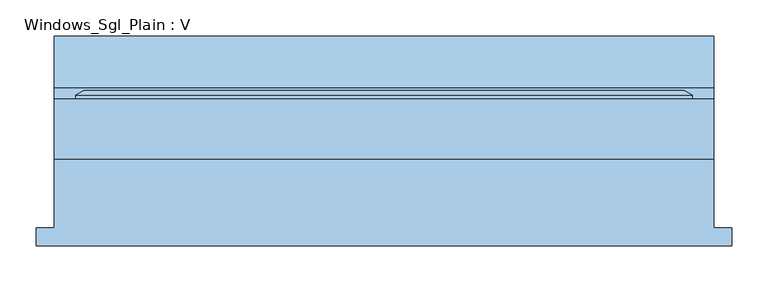
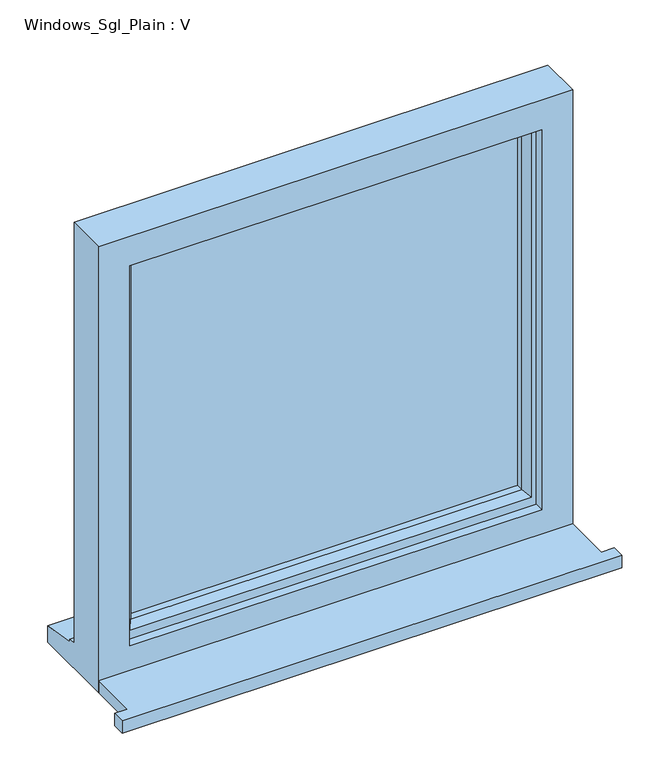
"""IFC4 building model written with IfcOpenShell, lengths in millimetres: window geometry, Windows_Sgl_Plain : V."""

from ifc_helpers import new_model, si_unit, frame, origin, place, context, project, spatial, polyline, outline, extrude, faceted_brep, source, transform, mapped, element, save


def windows_sgl_plain_v_28d0678b(model_context):
    return source(origin(), model_context, "Body", "SolidModel", [
        extrude(outline(polyline([(-482.2, -130.8434322), (-482.2, -105.8434322), (-457.2, -105.8434322), (-457.2, -10.2434322), (457.2, -10.2434322), (457.2, -105.8434322), (482.2, -105.8434322), (482.2, -130.8434322), (-482.2, -130.8434322)])), frame((0.0, 0.0, 1200.0), z_axis=(0.0, 0.0, 1.0), x_axis=(1.0, 0.0, 0.0)), (0.0, 0.0, 1.0), 25.0),
        faceted_brep([(-457.2, -10.2434322, 1200.0), (457.2, -10.2434322, 1200.0), (457.2, -10.2434322, 2110.0), (-457.2, -10.2434322, 2110.0), (-397.2, -10.2434322, 2050.0), (397.2, -10.2434322, 2050.0), (397.2, -10.2434322, 1275.0), (-397.2, -10.2434322, 1275.0), (-457.2, 72.7565678, 2110.0), (-457.2, 72.7565678, 1251.0), (-457.2, 87.7565678, 1249.68767), (-457.2, 87.7565678, 1244.7449676), (-457.2, 160.2565678, 1233.8088847), (-457.2, 160.2565678, 1200.0), (457.2, 72.7565678, 2110.0), (457.2, 72.7565678, 1251.0), (-417.2, 72.7565678, 2070.0), (-417.2, 72.7565678, 1263.0), (417.2, 72.7565678, 1263.0), (417.2, 72.7565678, 2070.0), (-417.2, 7.7565678, 2070.0), (-417.2, 7.7565678, 1263.0), (417.2, 7.7565678, 2070.0), (417.2, 7.7565678, 1263.0), (-397.2, 7.7565678, 2050.0), (-397.2, 7.7565678, 1275.0), (397.2, 7.7565678, 1275.0), (397.2, 7.7565678, 2050.0), (457.2, 160.2565678, 1200.0), (457.2, 160.2565678, 1233.8088847), (457.2, 87.7565678, 1244.7449676), (457.2, 87.7565678, 1249.68767)], [[[0, 1, 2, 3], [4, 5, 6, 7]], [[0, 3, 8, 9, 10, 11, 12, 13]], [[9, 8, 14, 15], [16, 17, 18, 19]], [[17, 16, 20, 21]], [[20, 22, 23, 21], [24, 25, 26, 27]], [[24, 4, 7, 25]], [[3, 2, 14, 8]], [[16, 19, 22, 20]], [[5, 4, 24, 27]], [[15, 14, 2, 1, 28, 29, 30, 31]], [[19, 18, 23, 22]], [[5, 27, 26, 6]], [[28, 1, 0, 13]], [[29, 28, 13, 12]], [[30, 29, 12, 11]], [[31, 30, 11, 10]], [[15, 31, 10, 9]], [[21, 23, 18, 17]], [[7, 6, 26, 25]]]),
        extrude(outline(polyline([(387.2, 36.7565678), (-387.2, 36.7565678), (-387.2, 60.7565678), (387.2, 60.7565678), (387.2, 36.7565678)])), frame((0.0, 0.0, 1293.0), z_axis=(0.0, 0.0, 1.0), x_axis=(1.0, 0.0, 0.0)), (0.0, 0.0, 1.0), 747.0),
        faceted_brep([(-427.2, 72.7565678, 2080.0), (-427.2, 78.5300705, 2080.0), (-427.2, 78.5300705, 1253.0), (-427.2, 72.7565678, 1253.0), (-417.2, 7.7565678, 2070.0), (-417.2, 72.7565678, 2070.0), (-417.2, 72.7565678, 1263.0), (-417.2, 7.7565678, 1263.0), (-377.2, 22.2494677, 2030.0), (-387.3480377, 7.7565678, 2040.1480377), (-387.3480377, 7.7565678, 1292.8519623), (-377.2, 22.2494677, 1303.0), (-377.2, 36.7565678, 2030.0), (-377.2, 36.7565678, 1303.0), (-387.2, 60.7565678, 2040.0), (-387.2, 36.7565678, 2040.0), (-387.2, 36.7565678, 1293.0), (-387.2, 60.7565678, 1293.0), (-377.2, 78.5300705, 2030.0), (-377.2, 60.7565678, 2030.0), (-377.2, 60.7565678, 1303.0), (-377.2, 78.5300705, 1303.0), (-394.6457548, 84.3035732, 2047.4457548), (-394.6457548, 84.3035732, 1285.5542452), (-416.4153903, 84.3035732, 2069.2153903), (-416.4153903, 84.3035732, 1263.7846097), (427.2, 78.5300705, 1253.0), (427.2, 72.7565678, 1253.0), (417.2, 72.7565678, 1263.0), (417.2, 7.7565678, 1263.0), (387.3480377, 7.7565678, 1292.8519623), (377.2, 22.2494677, 1303.0), (377.2, 36.7565678, 1303.0), (387.2, 36.7565678, 1293.0), (387.2, 60.7565678, 1293.0), (377.2, 60.7565678, 1303.0), (377.2, 78.5300705, 1303.0), (394.6457548, 84.3035732, 1285.5542452), (416.4153903, 84.3035732, 1263.7846097), (427.2, 78.5300705, 2080.0), (427.2, 72.7565678, 2080.0), (417.2, 72.7565678, 2070.0), (417.2, 7.7565678, 2070.0), (387.3480377, 7.7565678, 2040.1480377), (377.2, 22.2494677, 2030.0), (377.2, 36.7565678, 2030.0), (387.2, 36.7565678, 2040.0), (387.2, 60.7565678, 2040.0), (377.2, 60.7565678, 2030.0), (377.2, 78.5300705, 2030.0), (394.6457548, 84.3035732, 2047.4457548), (416.4153903, 84.3035732, 2069.2153903)], [[[0, 1, 2, 3]], [[4, 5, 6, 7]], [[8, 9, 10, 11]], [[12, 8, 11, 13]], [[14, 15, 16, 17]], [[18, 19, 20, 21]], [[22, 18, 21, 23]], [[1, 24, 25, 2]], [[3, 2, 26, 27]], [[7, 6, 28, 29]], [[11, 10, 30, 31]], [[13, 11, 31, 32]], [[17, 16, 33, 34]], [[21, 20, 35, 36]], [[23, 21, 36, 37]], [[2, 25, 38, 26]], [[27, 26, 39, 40]], [[29, 28, 41, 42]], [[31, 30, 43, 44]], [[32, 31, 44, 45]], [[34, 33, 46, 47]], [[36, 35, 48, 49]], [[37, 36, 49, 50]], [[26, 38, 51, 39]], [[40, 39, 1, 0]], [[3, 27, 40, 0], [5, 41, 28, 6]], [[42, 41, 5, 4]], [[7, 29, 42, 4], [9, 43, 30, 10]], [[44, 43, 9, 8]], [[45, 44, 8, 12]], [[15, 46, 33, 16], [13, 32, 45, 12]], [[47, 46, 15, 14]], [[17, 34, 47, 14], [19, 48, 35, 20]], [[49, 48, 19, 18]], [[50, 49, 18, 22]], [[24, 51, 38, 25], [23, 37, 50, 22]], [[39, 51, 24, 1]]]),
    ])


if __name__ == "__main__":
    model = new_model("IFC4")
    model_context = context("Model", 3, world=origin())
    ifc_project = project(units=[si_unit("LENGTHUNIT", "METRE", prefix="MILLI")], contexts=[model_context])
    site = spatial("IfcSite", under=ifc_project)
    building = spatial("IfcBuilding", under=site)
    placement = place(None, origin())
    windows_sgl_plain_v_shape = windows_sgl_plain_v_28d0678b(model_context)
    element("IfcWindow", 1, ObjectType="Windows_Sgl_Plain : V", at=placement, inside=building, context=model_context, shape_type="MappedRepresentation", body=[
        mapped(windows_sgl_plain_v_shape, transform((0.0, 0.0, 0.0), x_axis=(1.0, 0.0, 0.0), y_axis=(0.0, 1.0, 0.0), z_axis=(0.0, 0.0, 1.0))),
    ])
    save(model, "model.ifc")

# Revit data of these elements
# Type "Windows_Sgl_Plain : V"
#   Type Mark = "58"
#   Operation = "SinglePanel"
#   Construction Type Id = "SGL"
#   Manufacturer = "Revit"
#   Keynote = "L10"
#   Analytic Construction = "Large single-glazed windows"
#   Wrap Layers (Ext) from Ext = 0.336286 ft
#   Wrap Layers (Int) from Ext = 0.582349 ft
#   Window Board Projection = 0.082021 ft
#   Window Board Extension = 0.082021 ft
#   Visual Light Transmittance = 0.9
#   Solar Heat Gain Coefficient = 0.86
#   Rough Width = 3.0 ft
#   Rough Height = 2.985564 ft
#   Height = 2.985564 ft
#   Width = 3.0 ft
#   Heat Transfer Coefficient (U) = 5.5617 W/(m²·K)
#   Glazing Thickness = 0.07874 ft
#   FrameOffset - External = 0.164042 ft
#   Frame Depth = 0.213255 ft
#   Default Head Height = 6.922572 ft
#   Cill Depth = 0.287073 ft
#   Cavity Closer Width = 0.164042 ft
#   Cavity Closer Offset from Ext = 0.336286 ft
#   Cavity Closer Depth = 0.278871 ft
#   Vis - Cavity Closers = yes
#   Define Thermal Properties by = 1
#   Material Trim = Window Frame
#   Material Glass = Glass
#   Material Frame = Window Frame
#   Wall Closure = (empty or 0)
# Element 1 (IfcWindow, "Windows_Sgl_Plain : V")
#   Materials on its faces: "Window Frame", "Glass"
# Materials
#   "Window Frame": colour RGB 249 249 249, transparency 0, Keynote = "L10", Cost = 0
#   "Glass": class "Glass", colour RGB 0 128 192, transparency 0.9, Description = "Soda Lime Glass", Cost = 0
